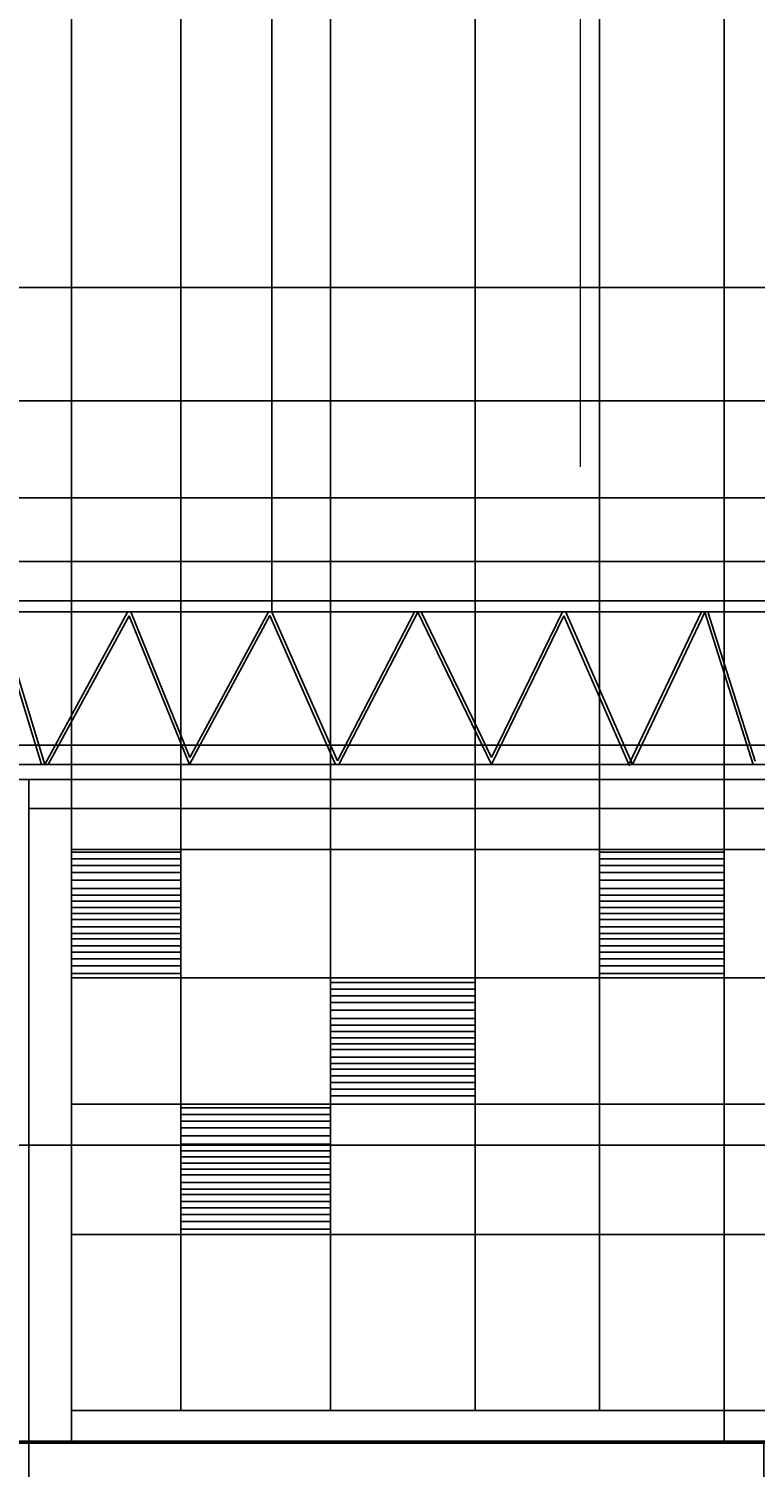
# Model space of a CAD drawing. Units: inches. Extents: x -32109 to 33221, y -19197 to 7608.
# Tile 10 of 25: x -11787 to -9406, y -2204 to 2510. Entities that reach past the tile are written whole.
import ezdxf

# ---------------------------------------------------------------- set-up
doc = ezdxf.new("R2010")
doc.units = ezdxf.units.IN
doc.header["$MEASUREMENT"] = 0
for name, color, linetype, lineweight in [('A-ANNO-DIMS', 2, 'Continuous', 18), ('A-ANNO-NOTE', 2, 'Continuous', 18), ('A-ELEV', 7, 'Continuous', 25)]:
    doc.layers.add(name, color=color, linetype=linetype, lineweight=lineweight)
doc.styles.get("Standard").update_dxf_attribs({"font": 'arial.ttf'})
doc.dimstyles.get("Standard").update_dxf_attribs({"dimtxt": 0.18, "dimasz": 0.18, "dimexe": 0.18, "dimexo": 0.0625, "dimgap": 0.09, "dimtad": 0, "dimtih": 1, "dimtoh": 1, "dimdec": 4, "dimzin": 0, "dimdsep": 46, "dimtxsty": 'Standard', "dimcen": 0.09, "dimadec": 0, "dimazin": 0, "dimtfac": 1, "dimtdec": 4, "dimtofl": 0, "dimtmove": 0, "dimatfit": 3, "dimfxl": 1, "dimtolj": 1, "dimtzin": 0, "dimarcsym": 0})

# ---------------------------------------------------------------- blocks, each defined once
blk = doc.blocks.new('*D10')
at = {"layer": 'A-ANNO-DIMS', "color": 0, "lineweight": -2, "transparency": 16777216}
for p, q in [((-18512.6, -110.2), (-18512.6, 5772)), ((-18512.5, 5771.8), (-202.1, 5771.8)), ((18109.1, 5771.8), (-201.2, 5771.8)), ((18109.3, -101.5), (18109.3, 5772))]:
    blk.add_line(p, q, dxfattribs=at)
at = {"layer": 'A-ANNO-DIMS', "color": 0, "transparency": 16777216}
for points in [[(-18512.5, 5771.9), (-18512.5, 5771.8), (-18512.6, 5771.8)], [(18109.1, 5771.9), (18109.1, 5771.8), (18109.3, 5771.8)]]:
    blk.add_solid(points, dxfattribs=at)
at = {"layer": 'Defpoints', "color": 0, "transparency": 16777216}
for p in [(18109.3, 5771.8), (-18512.6, -110.2), (18109.3, -101.6)]:
    blk.add_point(p, dxfattribs=at)
at = {"layer": 'A-ANNO-DIMS', "color": 0, "transparency": 16777216, "insert": (-201.7, 5771.8), "char_height": 0.18, "attachment_point": 5}
blk.add_mtext('\\A1;36622', dxfattribs=at)
blk = doc.blocks.new('*D11')
at = {"layer": 'A-ANNO-DIMS', "color": 0, "lineweight": -2, "transparency": 16777216}
for p, q in [((14509.6, 1705.2), (25710.6, 1705.2)), ((25710.5, 1705), (25710.5, -209.6)), ((25710.5, -2124.6), (25710.5, -210)), ((-18512.6, -2124.8), (25710.6, -2124.8))]:
    blk.add_line(p, q, dxfattribs=at)
at = {"layer": 'A-ANNO-DIMS', "color": 0, "transparency": 16777216}
for points in [[(25710.4, 1705), (25710.5, 1705), (25710.5, 1705.2)], [(25710.4, -2124.6), (25710.5, -2124.6), (25710.5, -2124.8)]]:
    blk.add_solid(points, dxfattribs=at)
at = {"layer": 'Defpoints', "color": 0, "transparency": 16777216}
for p in [(14509.6, 1705.2), (-18512.6, -2124.8), (25710.5, -2124.8)]:
    blk.add_point(p, dxfattribs=at)
at = {"layer": 'A-ANNO-DIMS', "color": 0, "transparency": 16777216, "insert": (25710.5, -209.8), "char_height": 0.18, "attachment_point": 5}
blk.add_mtext('\\A1;3830', dxfattribs=at)
blk = doc.blocks.new('*D21')
at = {"layer": 'A-ANNO-DIMS', "color": 0, "lineweight": -2, "transparency": 16777216}
for p, q in [((-5532.2, -1149.2), (-24362, -1149.2)), ((-24361.8, -1149.4), (-24361.8, -1636.8)), ((-24361.8, -2124.6), (-24361.8, -1637.2)), ((-5677.1, -2124.8), (-24362, -2124.8))]:
    blk.add_line(p, q, dxfattribs=at)
at = {"layer": 'A-ANNO-DIMS', "color": 0, "transparency": 16777216}
for points in [[(-24361.8, -1149.4), (-24361.8, -1149.4), (-24361.8, -1149.2)], [(-24361.8, -2124.6), (-24361.8, -2124.6), (-24361.8, -2124.8)]]:
    blk.add_solid(points, dxfattribs=at)
at = {"layer": 'Defpoints', "color": 0, "transparency": 16777216}
for p in [(-24361.8, -1149.2), (-5532.1, -1149.2), (-5677.1, -2124.8)]:
    blk.add_point(p, dxfattribs=at)
at = {"layer": 'A-ANNO-DIMS', "color": 0, "transparency": 16777216, "insert": (-24361.8, -1637), "char_height": 0.18, "attachment_point": 5}
blk.add_mtext('\\A1;975.6', dxfattribs=at)
blk = doc.blocks.new('*D27')
at = {"layer": 'A-ANNO-DIMS', "color": 0, "lineweight": -2, "transparency": 16777216}
for p, q in [((-11787, -2124.9), (-11787, -5429.7)), ((-9378.4, -2124.9), (-9378.4, -5429.7)), ((-11786.8, -5429.6), (-10583.2, -5429.6)), ((-9378.6, -5429.6), (-10582.2, -5429.6))]:
    blk.add_line(p, q, dxfattribs=at)
at = {"layer": 'A-ANNO-DIMS', "color": 0, "transparency": 16777216}
for points in [[(-11786.8, -5429.5), (-11786.8, -5429.6), (-11787, -5429.6)], [(-9378.6, -5429.5), (-9378.6, -5429.6), (-9378.4, -5429.6)]]:
    blk.add_solid(points, dxfattribs=at)
at = {"layer": 'Defpoints', "color": 0, "transparency": 16777216}
for p in [(-11787, -2124.8), (-9378.4, -2124.8), (-9378.4, -5429.6)]:
    blk.add_point(p, dxfattribs=at)
at = {"layer": 'A-ANNO-DIMS', "color": 0, "transparency": 16777216, "insert": (-10582.7, -5429.6), "char_height": 0.18, "attachment_point": 5}
blk.add_mtext('\\A1;2408.6', dxfattribs=at)
blk = doc.blocks.new('*D39')
at = {"layer": 'A-ANNO-DIMS', "color": 0, "lineweight": -2, "transparency": 16777216}
for p, q in [((-7375.9, 1290), (-24362, 1290)), ((-24361.8, 1289.8), (-24361.8, -414)), ((-24361.8, -2118.3), (-24361.8, -414.4)), ((-7754.5, -2118.4), (-24362, -2118.4))]:
    blk.add_line(p, q, dxfattribs=at)
at = {"layer": 'A-ANNO-DIMS', "color": 0, "transparency": 16777216}
for points in [[(-24361.8, 1289.8), (-24361.8, 1289.8), (-24361.8, 1290)], [(-24361.8, -2118.3), (-24361.8, -2118.3), (-24361.8, -2118.4)]]:
    blk.add_solid(points, dxfattribs=at)
at = {"layer": 'Defpoints', "color": 0, "transparency": 16777216}
for p in [(-7375.9, 1290), (-24361.8, -2118.4), (-7754.4, -2118.4)]:
    blk.add_point(p, dxfattribs=at)
at = {"layer": 'A-ANNO-DIMS', "color": 0, "transparency": 16777216, "insert": (-24361.8, -414.2), "char_height": 0.18, "attachment_point": 5}
blk.add_mtext('\\A1;3408.5', dxfattribs=at)
blk = doc.blocks.new('*D40')
at = {"layer": 'A-ANNO-DIMS', "color": 0, "lineweight": -2, "transparency": 16777216}
for p, q in [((-5445.1, 973), (-24362, 973)), ((-24361.8, 972.8), (-24361.8, -575.7)), ((-24361.8, -2124.6), (-24361.8, -576.1)), ((-5677.1, -2124.8), (-24362, -2124.8))]:
    blk.add_line(p, q, dxfattribs=at)
at = {"layer": 'A-ANNO-DIMS', "color": 0, "transparency": 16777216}
for points in [[(-24361.8, 972.8), (-24361.8, 972.8), (-24361.8, 973)], [(-24361.8, -2124.6), (-24361.8, -2124.6), (-24361.8, -2124.8)]]:
    blk.add_solid(points, dxfattribs=at)
at = {"layer": 'Defpoints', "color": 0, "transparency": 16777216}
for p in [(-5445, 973), (-24361.8, -2124.8), (-5677.1, -2124.8)]:
    blk.add_point(p, dxfattribs=at)
at = {"layer": 'A-ANNO-DIMS', "color": 0, "transparency": 16777216, "insert": (-24361.8, -575.9), "char_height": 0.18, "attachment_point": 5}
blk.add_mtext('\\A1;3098', dxfattribs=at)
blk = doc.blocks.new('*D41')
at = {"layer": 'A-ANNO-DIMS', "color": 0, "lineweight": -2, "transparency": 16777216}
for p, q in [((-651, 162.2), (-24362, 162.2)), ((-24361.8, 162), (-24361.8, -981.1)), ((-24361.8, -2124.6), (-24361.8, -981.5)), ((-651, -2124.8), (-24362, -2124.8))]:
    blk.add_line(p, q, dxfattribs=at)
at = {"layer": 'A-ANNO-DIMS', "color": 0, "transparency": 16777216}
for points in [[(-24361.8, 162), (-24361.8, 162), (-24361.8, 162.2)], [(-24361.8, -2124.6), (-24361.8, -2124.6), (-24361.8, -2124.8)]]:
    blk.add_solid(points, dxfattribs=at)
at = {"layer": 'Defpoints', "color": 0, "transparency": 16777216}
for p in [(-651, 162.2), (-24361.8, -2124.8), (-651, -2124.8)]:
    blk.add_point(p, dxfattribs=at)
at = {"layer": 'A-ANNO-DIMS', "color": 0, "transparency": 16777216, "insert": (-24361.8, -981.3), "char_height": 0.18, "attachment_point": 5}
blk.add_mtext('\\A1;2287', dxfattribs=at)
blk = doc.blocks.new('*D43')
at = {"layer": 'A-ANNO-DIMS', "color": 0, "lineweight": -2, "transparency": 16777216}
for p, q in [((-7375.9, 99.1), (-24362, 99.1)), ((-24361.8, 98.9), (-24361.8, -1009.5)), ((-24361.8, -2118.3), (-24361.8, -1009.8)), ((-7754.5, -2118.4), (-24362, -2118.4))]:
    blk.add_line(p, q, dxfattribs=at)
at = {"layer": 'A-ANNO-DIMS', "color": 0, "transparency": 16777216}
for points in [[(-24361.8, 98.9), (-24361.8, 98.9), (-24361.8, 99.1)], [(-24361.8, -2118.3), (-24361.8, -2118.3), (-24361.8, -2118.4)]]:
    blk.add_solid(points, dxfattribs=at)
at = {"layer": 'Defpoints', "color": 0, "transparency": 16777216}
for p in [(-7375.9, 99.1), (-24361.8, -2118.4), (-7754.4, -2118.4)]:
    blk.add_point(p, dxfattribs=at)
at = {"layer": 'A-ANNO-DIMS', "color": 0, "transparency": 16777216, "insert": (-24361.8, -1009.7), "char_height": 0.18, "attachment_point": 5}
blk.add_mtext('\\A1;2217.5', dxfattribs=at)
blk = doc.blocks.new('*D44')
at = {"layer": 'A-ANNO-DIMS', "color": 0, "lineweight": -2, "transparency": 16777216}
for p, q in [((-12501.4, 764.2), (-12501.4, 5772)), ((-12501.2, 5771.8), (-9939, 5771.8)), ((-7376.1, 5771.8), (-9938.3, 5771.8)), ((-7375.9, 764.2), (-7375.9, 5772))]:
    blk.add_line(p, q, dxfattribs=at)
at = {"layer": 'A-ANNO-DIMS', "color": 0, "transparency": 16777216}
for points in [[(-12501.2, 5771.9), (-12501.2, 5771.8), (-12501.4, 5771.8)], [(-7376.1, 5771.9), (-7376.1, 5771.8), (-7375.9, 5771.8)]]:
    blk.add_solid(points, dxfattribs=at)
at = {"layer": 'Defpoints', "color": 0, "transparency": 16777216}
for p in [(-7375.9, 5771.8), (-12501.4, 764.2), (-7375.9, 764.2)]:
    blk.add_point(p, dxfattribs=at)
at = {"layer": 'A-ANNO-DIMS', "color": 0, "transparency": 16777216, "insert": (-9938.6, 5771.8), "char_height": 0.18, "attachment_point": 5}
blk.add_mtext('\\A1;5125', dxfattribs=at)
blk = doc.blocks.new('*D45')
at = {"layer": 'A-ANNO-DIMS', "color": 0, "lineweight": -2, "transparency": 16777216}
for p, q in [((-11898.6, 599), (-11898.6, 5772)), ((-11898.4, 5771.8), (-11444.9, 5771.8)), ((-10990.6, 5771.8), (-11444.1, 5771.8)), ((-10990.5, 598.1), (-10990.5, 5772))]:
    blk.add_line(p, q, dxfattribs=at)
at = {"layer": 'A-ANNO-DIMS', "color": 0, "transparency": 16777216}
for points in [[(-11898.4, 5771.9), (-11898.4, 5771.8), (-11898.6, 5771.8)], [(-10990.6, 5771.9), (-10990.6, 5771.8), (-10990.5, 5771.8)]]:
    blk.add_solid(points, dxfattribs=at)
at = {"layer": 'Defpoints', "color": 0, "transparency": 16777216}
for p in [(-10990.5, 5771.8), (-11898.6, 598.9), (-10990.5, 598)]:
    blk.add_point(p, dxfattribs=at)
at = {"layer": 'A-ANNO-DIMS', "color": 0, "transparency": 16777216, "insert": (-11444.5, 5771.8), "char_height": 0.18, "attachment_point": 5}
blk.add_mtext('\\A1;908.1', dxfattribs=at)
blk = doc.blocks.new('*D48')
at = {"layer": 'A-ANNO-DIMS', "color": 0, "lineweight": -2, "transparency": 16777216}
for p, q in [((-11646.5, -179.6), (-11646.5, 5772)), ((-11646.3, 5771.8), (-11468.1, 5771.8)), ((-11288.9, 5771.8), (-11467.2, 5771.8)), ((-11288.8, -179.6), (-11288.8, 5772))]:
    blk.add_line(p, q, dxfattribs=at)
at = {"layer": 'A-ANNO-DIMS', "color": 0, "transparency": 16777216}
for points in [[(-11646.3, 5771.9), (-11646.3, 5771.8), (-11646.5, 5771.8)], [(-11288.9, 5771.9), (-11288.9, 5771.8), (-11288.8, 5771.8)]]:
    blk.add_solid(points, dxfattribs=at)
at = {"layer": 'Defpoints', "color": 0, "transparency": 16777216}
for p in [(-11288.8, 5771.8), (-11646.5, -179.7), (-11288.8, -179.7)]:
    blk.add_point(p, dxfattribs=at)
at = {"layer": 'A-ANNO-DIMS', "color": 0, "transparency": 16777216, "insert": (-11467.6, 5771.8), "char_height": 0.18, "attachment_point": 5}
blk.add_mtext('\\A1;357.75', dxfattribs=at)
blk = doc.blocks.new('*D49')
at = {"layer": 'A-ANNO-DIMS', "color": 0, "lineweight": -2, "transparency": 16777216}
for p, q in [((-11288.8, -179.6), (-11288.8, 5772)), ((-11288.6, 5771.8), (-11043.7, 5771.8)), ((-10798.1, 5771.8), (-11042.9, 5771.8)), ((-10797.9, -179.6), (-10797.9, 5772))]:
    blk.add_line(p, q, dxfattribs=at)
at = {"layer": 'A-ANNO-DIMS', "color": 0, "transparency": 16777216}
for points in [[(-11288.6, 5771.9), (-11288.6, 5771.8), (-11288.8, 5771.8)], [(-10798.1, 5771.9), (-10798.1, 5771.8), (-10797.9, 5771.8)]]:
    blk.add_solid(points, dxfattribs=at)
at = {"layer": 'Defpoints', "color": 0, "transparency": 16777216}
for p in [(-10797.9, 5771.8), (-11288.8, -179.7), (-10797.9, -179.7)]:
    blk.add_point(p, dxfattribs=at)
at = {"layer": 'A-ANNO-DIMS', "color": 0, "transparency": 16777216, "insert": (-11043.3, 5771.8), "char_height": 0.18, "attachment_point": 5}
blk.add_mtext('\\A1;490.9', dxfattribs=at)
blk = doc.blocks.new('*D50')
at = {"layer": 'A-ANNO-DIMS', "color": 0, "lineweight": -2, "transparency": 16777216}
for p, q in [((-10797.9, -179.6), (-10797.9, 5772)), ((-10797.7, 5771.8), (-10561.2, 5771.8)), ((-10323.8, 5771.8), (-10560.4, 5771.8)), ((-10323.7, -179.6), (-10323.7, 5772))]:
    blk.add_line(p, q, dxfattribs=at)
at = {"layer": 'A-ANNO-DIMS', "color": 0, "transparency": 16777216}
for points in [[(-10797.7, 5771.9), (-10797.7, 5771.8), (-10797.9, 5771.8)], [(-10323.8, 5771.9), (-10323.8, 5771.8), (-10323.7, 5771.8)]]:
    blk.add_solid(points, dxfattribs=at)
at = {"layer": 'Defpoints', "color": 0, "transparency": 16777216}
for p in [(-10323.7, 5771.8), (-10797.9, -179.7), (-10323.7, -179.7)]:
    blk.add_point(p, dxfattribs=at)
at = {"layer": 'A-ANNO-DIMS', "color": 0, "transparency": 16777216, "insert": (-10560.8, 5771.8), "char_height": 0.18, "attachment_point": 5}
blk.add_mtext('\\A1;474.2', dxfattribs=at)
blk = doc.blocks.new('*D51')
at = {"layer": 'A-ANNO-DIMS', "color": 0, "lineweight": -2, "transparency": 16777216}
for p, q in [((-10323.7, -179.6), (-10323.7, 5772)), ((-10323.5, 5771.8), (-10120.2, 5771.8)), ((-9916.2, 5771.8), (-10119.4, 5771.8)), ((-9916, -179.6), (-9916, 5772))]:
    blk.add_line(p, q, dxfattribs=at)
at = {"layer": 'A-ANNO-DIMS', "color": 0, "transparency": 16777216}
for points in [[(-10323.5, 5771.9), (-10323.5, 5771.8), (-10323.7, 5771.8)], [(-9916.2, 5771.9), (-9916.2, 5771.8), (-9916, 5771.8)]]:
    blk.add_solid(points, dxfattribs=at)
at = {"layer": 'Defpoints', "color": 0, "transparency": 16777216}
for p in [(-9916, 5771.8), (-10323.7, -179.7), (-9916, -179.7)]:
    blk.add_point(p, dxfattribs=at)
at = {"layer": 'A-ANNO-DIMS', "color": 0, "transparency": 16777216, "insert": (-10119.8, 5771.8), "char_height": 0.18, "attachment_point": 5}
blk.add_mtext('\\A1;407.7', dxfattribs=at)
blk = doc.blocks.new('*D52')
at = {"layer": 'A-ANNO-DIMS', "color": 0, "lineweight": -2, "transparency": 16777216}
for p, q in [((-9916, -179.6), (-9916, 5772)), ((-9915.8, 5771.8), (-9712.6, 5771.8)), ((-9508.5, 5771.8), (-9711.8, 5771.8)), ((-9508.3, -179.6), (-9508.3, 5772))]:
    blk.add_line(p, q, dxfattribs=at)
at = {"layer": 'A-ANNO-DIMS', "color": 0, "transparency": 16777216}
for points in [[(-9915.8, 5771.9), (-9915.8, 5771.8), (-9916, 5771.8)], [(-9508.5, 5771.9), (-9508.5, 5771.8), (-9508.3, 5771.8)]]:
    blk.add_solid(points, dxfattribs=at)
at = {"layer": 'Defpoints', "color": 0, "transparency": 16777216}
for p in [(-9508.3, 5771.8), (-9916, -179.7), (-9508.3, -179.7)]:
    blk.add_point(p, dxfattribs=at)
at = {"layer": 'A-ANNO-DIMS', "color": 0, "transparency": 16777216, "insert": (-9712.2, 5771.8), "char_height": 0.18, "attachment_point": 5}
blk.add_mtext('\\A1;407.7', dxfattribs=at)
blk = doc.blocks.new('*D53')
at = {"layer": 'A-ANNO-DIMS', "color": 0, "lineweight": -2, "transparency": 16777216}
for p, q in [((-9508.3, -179.7), (25710.6, -179.7)), ((25710.5, -179.9), (25710.5, -389.7)), ((25710.5, -600), (25710.5, -390.1)), ((-9508.3, -600.2), (25710.6, -600.2))]:
    blk.add_line(p, q, dxfattribs=at)
at = {"layer": 'A-ANNO-DIMS', "color": 0, "transparency": 16777216}
for points in [[(25710.4, -179.9), (25710.5, -179.9), (25710.5, -179.7)], [(25710.4, -600), (25710.5, -600), (25710.5, -600.2)]]:
    blk.add_solid(points, dxfattribs=at)
at = {"layer": 'Defpoints', "color": 0, "transparency": 16777216}
for p in [(-9508.3, -179.7), (-9508.3, -600.2), (25710.5, -600.2)]:
    blk.add_point(p, dxfattribs=at)
at = {"layer": 'A-ANNO-DIMS', "color": 0, "transparency": 16777216, "insert": (25710.5, -389.9), "char_height": 0.18, "attachment_point": 5}
blk.add_mtext('\\A1;420.5', dxfattribs=at)
blk = doc.blocks.new('*D54')
at = {"layer": 'A-ANNO-DIMS', "color": 0, "lineweight": -2, "transparency": 16777216}
for p, q in [((-9508.3, -600.2), (25710.6, -600.2)), ((25710.5, -600.3), (25710.5, -806.8)), ((25710.5, -1013.7), (25710.5, -807.2)), ((-9508.3, -1013.9), (25710.6, -1013.9))]:
    blk.add_line(p, q, dxfattribs=at)
at = {"layer": 'A-ANNO-DIMS', "color": 0, "transparency": 16777216}
for points in [[(25710.4, -600.3), (25710.5, -600.3), (25710.5, -600.2)], [(25710.4, -1013.7), (25710.5, -1013.7), (25710.5, -1013.9)]]:
    blk.add_solid(points, dxfattribs=at)
at = {"layer": 'Defpoints', "color": 0, "transparency": 16777216}
for p in [(-9508.3, -600.2), (-9508.3, -1013.9), (25710.5, -1013.9)]:
    blk.add_point(p, dxfattribs=at)
at = {"layer": 'A-ANNO-DIMS', "color": 0, "transparency": 16777216, "insert": (25710.5, -807), "char_height": 0.18, "attachment_point": 5}
blk.add_mtext('\\A1;413.7', dxfattribs=at)
blk = doc.blocks.new('*D55')
at = {"layer": 'A-ANNO-DIMS', "color": 0, "lineweight": -2, "transparency": 16777216}
for p, q in [((-9508.3, -1013.9), (25710.6, -1013.9)), ((25710.5, -1014.1), (25710.5, -1227.7)), ((25710.5, -1441.6), (25710.5, -1228)), ((-9508.3, -1441.8), (25710.6, -1441.8))]:
    blk.add_line(p, q, dxfattribs=at)
at = {"layer": 'A-ANNO-DIMS', "color": 0, "transparency": 16777216}
for points in [[(25710.4, -1014.1), (25710.5, -1014.1), (25710.5, -1013.9)], [(25710.4, -1441.6), (25710.5, -1441.6), (25710.5, -1441.8)]]:
    blk.add_solid(points, dxfattribs=at)
at = {"layer": 'Defpoints', "color": 0, "transparency": 16777216}
for p in [(-9508.3, -1013.9), (-9508.3, -1441.8), (25710.5, -1441.8)]:
    blk.add_point(p, dxfattribs=at)
at = {"layer": 'A-ANNO-DIMS', "color": 0, "transparency": 16777216, "insert": (25710.5, -1227.9), "char_height": 0.18, "attachment_point": 5}
blk.add_mtext('\\A1;427.9', dxfattribs=at)
blk = doc.blocks.new('*D56')
at = {"layer": 'A-ANNO-DIMS', "color": 0, "lineweight": -2, "transparency": 16777216}
for p, q in [((-9508.3, -1441.8), (25710.6, -1441.8)), ((25710.5, -1442), (25710.5, -1730.1)), ((25710.5, -2018.6), (25710.5, -1730.5)), ((-9508.3, -2018.8), (25710.6, -2018.8))]:
    blk.add_line(p, q, dxfattribs=at)
at = {"layer": 'A-ANNO-DIMS', "color": 0, "transparency": 16777216}
for points in [[(25710.4, -1442), (25710.5, -1442), (25710.5, -1441.8)], [(25710.4, -2018.6), (25710.5, -2018.6), (25710.5, -2018.8)]]:
    blk.add_solid(points, dxfattribs=at)
at = {"layer": 'Defpoints', "color": 0, "transparency": 16777216}
for p in [(-9508.3, -1441.8), (-9508.3, -2018.8), (25710.5, -2018.8)]:
    blk.add_point(p, dxfattribs=at)
at = {"layer": 'A-ANNO-DIMS', "color": 0, "transparency": 16777216, "insert": (25710.5, -1730.3), "char_height": 0.18, "attachment_point": 5}
blk.add_mtext('\\A1;576.9', dxfattribs=at)
blk = doc.blocks.new('*D158')
at = {"layer": 'A-ANNO-DIMS', "color": 0, "lineweight": -2, "transparency": 16777216}
for p, q in [((5447.3, 1662.2), (-24362, 1662.2)), ((-24361.8, 1662), (-24361.8, -230.1)), ((-24361.8, -2122.6), (-24361.8, -230.5)), ((5279.2, -2122.7), (-24362, -2122.7))]:
    blk.add_line(p, q, dxfattribs=at)
at = {"layer": 'A-ANNO-DIMS', "color": 0, "transparency": 16777216}
for points in [[(-24361.8, 1662), (-24361.8, 1662), (-24361.8, 1662.2)], [(-24361.8, -2122.6), (-24361.8, -2122.6), (-24361.8, -2122.7)]]:
    blk.add_solid(points, dxfattribs=at)
at = {"layer": 'Defpoints', "color": 0, "transparency": 16777216}
for p in [(5447.3, 1662.2), (-24361.8, -2122.7), (5279.3, -2122.7)]:
    blk.add_point(p, dxfattribs=at)
at = {"layer": 'A-ANNO-DIMS', "color": 0, "transparency": 16777216, "insert": (-24361.8, -230.3), "char_height": 0.18, "attachment_point": 5}
blk.add_mtext('\\A1;3784.9', dxfattribs=at)

msp = doc.modelspace()

# ---------------------------------------------------------------- linework, layer by layer
at = {"layer": 'A-ANNO-NOTE'}
msp.add_line((-9978.983, 1074.546), (-9978.983, 3321.835), dxfattribs=at)
at = {"layer": 'A-ELEV'}
for p, q in [((-7375.878, 764.187), (-12501.359, 764.187)), ((-12501.359, 635.262), (-7375.878, 635.262)), ((-7375.878, 598.924), (-12501.359, 598.924)), ((-11745.213, 99.103), (-11894.24, 585.798)), ((-11734.663, 98.805), (-11887.589, 598.233)), ((-11463.311, 598.161), (-11734.663, 98.805)), ((-11458.442, 586.177), (-11723.119, 99.103)), ((-11260.397, 98.719), (-11458.442, 586.177)), ((-11259.112, 122.123), (-11452.827, 598.924)), ((-10996.478, 586.863), (-11260.397, 98.719)), ((-11001.325, 598.924), (-11259.112, 122.123)), ((-10781.453, 99.103), (-10996.478, 586.863)), ((-10775.54, 110.48), (-10990.458, 597.998)), ((-10522.635, 598.924), (-10775.54, 110.48)), ((-10511.813, 598.075), (-10770.361, 98.733)), ((-10270.238, 98.785), (-10511.813, 598.075)), ((-10270.215, 121.697), (-10501.115, 598.924)), ((-10033.096, 586.376), (-10270.238, 98.785)), ((-10038.113, 598.924), (-10270.215, 121.697)), ((-9817.937, 94.834), (-10033.096, 586.376)), ((-9808.777, 98.844), (-10027.351, 598.189)), ((-9582.176, 598.924), (-9817.808, 103.136)), ((-9571.422, 598.255), (-9808.777, 98.844)), ((-9413.342, 99.103), (-9571.422, 598.255)), ((-9406.073, 109.271), (-9561.144, 598.924)), ((-12501.359, 99.103), (-7375.878, 99.103)), ((-10770.361, 98.733), (-10770.524, 99.103)), ((-7375.878, 49.157), (-12501.359, 49.157)), ((-11787.012, -740.123), (-11787.012, 49.358)), ((-11787.012, 49.358), (-9673.873, 49.157)), ((-9426.582, 49.157), (-11469.599, 49.157)), ((-9378.383, -45.544), (-11787.012, -45.544)), ((-11646.505, -2124.791), (-11646.505, -179.679)), ((-11646.505, -179.679), (-9508.333, -179.679)), ((-11288.757, -2018.754), (-11288.757, -179.679)), ((-10797.892, -2018.754), (-10797.892, -179.679)), ((-10323.667, -2018.754), (-10323.667, -179.679)), ((-9916, -2018.754), (-9916, -179.679)), ((-9508.333, -179.679), (-9508.333, -2124.791)), ((-11646.505, -189.049), (-11288.757, -189.049)), ((-11646.505, -210.357), (-11288.757, -210.357)), ((-11646.505, -232.408), (-11288.757, -232.408)), ((-9918.243, -189.049), (-9508.333, -189.049)), ((-9918.243, -210.357), (-9508.333, -210.357)), ((-9918.243, -232.408), (-9508.333, -232.408)), ((-11646.505, -254.63), (-11288.757, -254.63)), ((-11646.505, -280.104), (-11288.757, -280.104)), ((-9918.243, -254.63), (-9508.333, -254.63)), ((-9918.243, -280.104), (-9508.333, -280.104)), ((-11646.505, -307.204), (-11288.757, -307.204)), ((-11646.505, -329.069), (-11288.757, -329.069)), ((-9918.243, -307.204), (-9508.333, -307.204)), ((-9918.243, -329.069), (-9508.333, -329.069)), ((-11646.505, -349.664), (-11288.757, -349.664)), ((-11646.505, -369.718), (-11288.757, -369.718)), ((-9918.243, -349.664), (-9508.333, -349.664)), ((-9918.243, -369.718), (-9508.333, -369.718)), ((-11646.505, -389.772), (-11288.757, -389.772)), ((-11646.505, -408.742), (-11288.757, -408.742)), ((-9918.243, -389.772), (-9508.333, -389.772)), ((-9918.243, -408.742), (-9508.333, -408.742)), ((-11646.505, -433.696), (-11288.757, -433.696)), ((-11646.505, -454.772), (-11288.757, -454.772)), ((-9918.243, -433.696), (-9508.333, -433.696)), ((-9918.243, -454.772), (-9508.333, -454.772)), ((-11646.505, -472.788), (-11288.757, -472.788)), ((-11646.505, -495.171), (-11288.757, -495.171)), ((-11646.505, -516.479), (-11288.757, -516.479)), ((-9918.243, -472.788), (-9508.333, -472.788)), ((-9918.243, -495.171), (-9508.333, -495.171)), ((-9918.243, -516.479), (-9508.333, -516.479)), ((-11646.505, -538.53), (-11288.757, -538.53)), ((-11646.505, -560.752), (-11288.757, -560.752)), ((-9918.243, -538.53), (-9508.333, -538.53)), ((-9918.243, -560.752), (-9508.333, -560.752)), ((-11646.505, -586.226), (-11288.757, -586.226)), ((-11646.505, -600.154), (-9508.333, -600.154)), ((-9918.243, -586.226), (-9508.333, -586.226)), ((-10797.892, -615.785), (-10323.667, -615.785)), ((-10797.892, -637.093), (-10323.667, -637.093)), ((-10797.892, -659.145), (-10323.667, -659.145)), ((-10797.892, -681.366), (-10323.667, -681.366)), ((-10797.892, -706.84), (-10323.667, -706.84)), ((-11787.012, -740.123), (-11787.012, -2124.791)), ((-10797.892, -733.94), (-10323.667, -733.94)), ((-10797.892, -755.805), (-10323.667, -755.805)), ((-10797.892, -776.401), (-10323.667, -776.401)), ((-10797.892, -796.454), (-10323.667, -796.454)), ((-10797.892, -816.508), (-10323.667, -816.508)), ((-10797.892, -835.478), (-10323.667, -835.478)), ((-10797.892, -860.433), (-10323.667, -860.433)), ((-10797.892, -881.508), (-10323.667, -881.508)), ((-10797.892, -899.525), (-10323.667, -899.525)), ((-10797.892, -921.907), (-10323.667, -921.907)), ((-10797.892, -943.215), (-10323.667, -943.215)), ((-10797.892, -965.267), (-10323.667, -965.267)), ((-10797.892, -987.488), (-10323.667, -987.488)), ((-11646.505, -1013.888), (-9508.333, -1013.888)), ((-11288.757, -1026.771), (-10797.892, -1026.771)), ((-11288.757, -1048.079), (-10797.892, -1048.079)), ((-11288.757, -1070.13), (-10797.892, -1070.13)), ((-11288.757, -1092.352), (-10797.892, -1092.352)), ((-11288.757, -1117.826), (-10797.892, -1117.826)), ((-11288.757, -1144.926), (-10797.892, -1144.926)), ((-11288.757, -1166.791), (-10797.892, -1166.791)), ((-11288.757, -1187.386), (-10797.892, -1187.386)), ((-11288.757, -1207.44), (-10797.892, -1207.44)), ((-11288.757, -1227.494), (-10797.892, -1227.494)), ((-11288.757, -1246.464), (-10797.892, -1246.464)), ((-11288.757, -1271.418), (-10797.892, -1271.418)), ((-11288.757, -1292.494), (-10797.892, -1292.494)), ((-11288.757, -1310.51), (-10797.892, -1310.51)), ((-11288.757, -1332.893), (-10797.892, -1332.893)), ((-11288.757, -1354.201), (-10797.892, -1354.201)), ((-11288.757, -1376.252), (-10797.892, -1376.252)), ((-11288.757, -1398.474), (-10797.892, -1398.474)), ((-11646.505, -1441.815), (-9508.333, -1441.815)), ((-11288.757, -1423.948), (-10797.892, -1423.948)), ((-11646.505, -2018.754), (-9508.333, -2018.754)), ((-18512.647, -2124.791), (1683.588, -2124.791)), ((-3437.624, -2124.791), (-10277.124, -2124.791))]:
    msp.add_line(p, q, dxfattribs=at)

# ---------------------------------------------------------------- dimensions: what is measured, and where the dimension line sits
at = {"layer": 'A-ANNO-DIMS'}
for base, p1, p2, override, picture, middle in [((18109.317, 5771.835), (-18512.647, -110.242), (18109.317, -101.6), {"dimdec": 0, "dimlfac": 1, "dimrnd": 0, "dimzin": 0, "dimdsep": 46, "dimlunit": 2}, '*D10', (-201.665, 5771.835)), ((-7375.878, 5771.835), (-12501.359, 764.187), (-7375.878, 764.187), {"dimdec": 0, "dimlfac": 1, "dimrnd": 0, "dimzin": 0, "dimdsep": 46, "dimlunit": 2}, '*D44', (-9938.618, 5771.835)), ((-10990.458, 5771.835), (-11898.56, 598.924), (-10990.458, 597.998), {"dimdec": 1, "dimlfac": 1, "dimrnd": 0, "dimzin": 0, "dimdsep": 46, "dimlunit": 2}, '*D45', (-11444.509, 5771.835)), ((-11288.757, 5771.835), (-11646.505, -179.679), (-11288.757, -179.679), {"dimdec": 2, "dimlfac": 1, "dimrnd": 0, "dimzin": 0, "dimdsep": 46, "dimlunit": 2}, '*D48', (-11467.631, 5771.835)), ((-10797.892, 5771.835), (-11288.757, -179.679), (-10797.892, -179.679), {"dimdec": 1, "dimlfac": 1, "dimrnd": 0, "dimzin": 0, "dimdsep": 46, "dimlunit": 2}, '*D49', (-11043.325, 5771.835)), ((-10323.667, 5771.835), (-10797.892, -179.679), (-10323.667, -179.679), {"dimdec": 1, "dimlfac": 1, "dimrnd": 0, "dimzin": 0, "dimdsep": 46, "dimlunit": 2}, '*D50', (-10560.78, 5771.835)), ((-9916, 5771.835), (-10323.667, -179.679), (-9916, -179.679), {"dimdec": 1, "dimlfac": 1, "dimrnd": 0, "dimzin": 0, "dimdsep": 46, "dimlunit": 2}, '*D51', (-10119.834, 5771.835)), ((-9508.333, 5771.835), (-9916, -179.679), (-9508.333, -179.679), {"dimdec": 1, "dimlfac": 1, "dimrnd": 0, "dimzin": 0, "dimdsep": 46, "dimlunit": 2}, '*D52', (-9712.167, 5771.835)), ((-9378.383, -5429.555), (-11787.012, -2124.791), (-9378.383, -2124.791), {"dimdec": 1, "dimlfac": 1, "dimrnd": 0, "dimzin": 0, "dimdsep": 46, "dimlunit": 2}, '*D27', (-10582.697, -5429.555))]:
    dim = msp.add_linear_dim(base=base, p1=p1, p2=p2, dimstyle='Standard', override=override, dxfattribs=at)
    dim.commit()
    dim.dimension.update_dxf_attribs({"geometry": picture, "text_midpoint": middle})
for base, p1, p2, override, picture, middle in [((25710.469, -2124.791), (14509.55, 1705.162), (-18512.647, -2124.791), {"dimdec": 0, "dimlfac": 1, "dimrnd": 0, "dimzin": 0, "dimdsep": 46, "dimlunit": 2}, '*D11', (25710.469, -209.814)), ((-24361.816, -2122.749), (5447.329, 1662.17), (5279.264, -2122.749), {"dimdec": 1, "dimlfac": 1, "dimrnd": 0, "dimzin": 0, "dimdsep": 46, "dimlunit": 2}, '*D158', (-24361.816, -230.29)), ((-24361.816, -2118.431), (-7375.878, 1290.029), (-7754.412, -2118.431), {"dimdec": 1, "dimlfac": 1, "dimrnd": 0, "dimzin": 0, "dimdsep": 46, "dimlunit": 2}, '*D39', (-24361.816, -414.201)), ((-24361.816, -2124.791), (-5445.024, 973.011), (-5677.079, -2124.791), {"dimdec": 0, "dimlfac": 1, "dimrnd": 0, "dimzin": 0, "dimdsep": 46, "dimlunit": 2}, '*D40', (-24361.816, -575.89)), ((-24361.816, -2124.791), (-650.959, 162.186), (-650.959, -2124.791), {"dimdec": 0, "dimlfac": 1, "dimrnd": 0, "dimzin": 0, "dimdsep": 46, "dimlunit": 2}, '*D41', (-24361.816, -981.302)), ((-24361.816, -2118.431), (-7375.878, 99.103), (-7754.412, -2118.431), {"dimdec": 1, "dimlfac": 1, "dimrnd": 0, "dimzin": 0, "dimdsep": 46, "dimlunit": 2}, '*D43', (-24361.816, -1009.664)), ((25710.469, -600.154), (-9508.333, -179.679), (-9508.333, -600.154), {"dimdec": 1, "dimlfac": 1, "dimrnd": 0, "dimzin": 0, "dimdsep": 46, "dimlunit": 2}, '*D53', (25710.469, -389.916)), ((25710.469, -1013.888), (-9508.333, -600.154), (-9508.333, -1013.888), {"dimdec": 1, "dimlfac": 1, "dimrnd": 0, "dimzin": 0, "dimdsep": 46, "dimlunit": 2}, '*D54', (25710.469, -807.021)), ((25710.469, -1441.815), (-9508.333, -1013.888), (-9508.333, -1441.815), {"dimdec": 1, "dimlfac": 1, "dimrnd": 0, "dimzin": 0, "dimdsep": 46, "dimlunit": 2}, '*D55', (25710.469, -1227.851)), ((-24361.816, -1149.23), (-5677.079, -2124.791), (-5532.101, -1149.23), {"dimdec": 1, "dimlfac": 1, "dimrnd": 0, "dimzin": 0, "dimdsep": 46, "dimlunit": 2}, '*D21', (-24361.816, -1637.01)), ((25710.469, -2018.754), (-9508.333, -1441.815), (-9508.333, -2018.754), {"dimdec": 1, "dimlfac": 1, "dimrnd": 0, "dimzin": 0, "dimdsep": 46, "dimlunit": 2}, '*D56', (25710.469, -1730.285))]:
    dim = msp.add_linear_dim(base=base, p1=p1, p2=p2, angle=90, dimstyle='Standard', override=override, dxfattribs=at)
    dim.commit()
    dim.dimension.update_dxf_attribs({"geometry": picture, "text_midpoint": middle})

doc.saveas('drawing.dxf')
